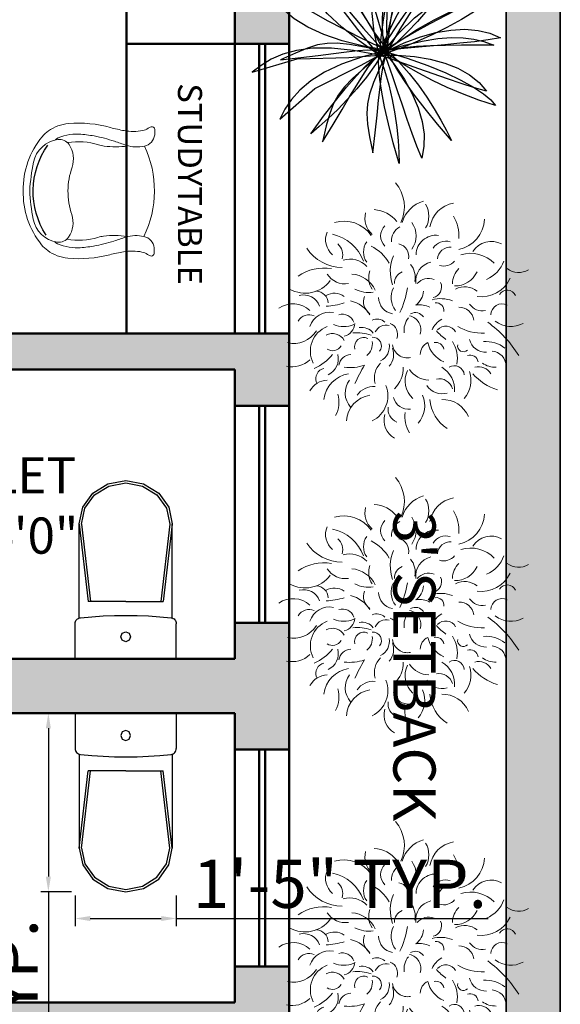
# Model space of a CAD drawing. Units: inches. Extents: x 2442 to 3851, y 589 to 2836.
# Tile 9 of 22: x 3004 to 3094, y 1717 to 1880. Entities that reach past the tile are written whole.
import ezdxf

# ---------------------------------------------------------------- set-up
doc = ezdxf.new("R2010")
doc.units = ezdxf.units.IN
for name, color, linetype, lineweight in [('A-ANNO-DIMS', 2, 'Continuous', 18), ('A-ANNO-TEXT', 7, 'Continuous', 18), ('A-AREA-IDEN', 7, 'Continuous', 18), ('A-FLOR-FIXT', 8, 'Continuous', 18), ('A-FURN', 8, 'Continuous', 18), ('A-WALL', 7, 'Continuous', 50), ('A-WALL-PATT', 8, 'Continuous', 13), ('C-PROP', 7, 'Continuous', 35), ('L-PLNT', 94, 'Continuous', 18)]:
    doc.layers.add(name, color=color, linetype=linetype, lineweight=lineweight)
for name, color, linetype in [('DIENHOA', 3, 'Continuous'), ('IFF-FURN-DETAIL', 250, 'Continuous'), ('SANTEH', 7, 'Continuous')]:
    doc.layers.add(name, color=color, linetype=linetype)
doc.styles.add('ATT', font='romans.shx')
doc.styles.get("Standard").update_dxf_attribs({"font": 'arial.ttf'})
doc.dimstyles.new('ISO-25', dxfattribs={"dimtxt": 8, "dimasz": 2.5, "dimexe": 1.25, "dimexo": 0.625, "dimtad": 1, "dimlunit": 3, "dimtxsty": 'Standard', "dimcen": 2.5, "dimadec": 0, "dimazin": 0, "dimtfac": 1, "dimtmove": 0, "dimatfit": 3, "dimfxl": 1, "dimarcsym": 0})

# ---------------------------------------------------------------- blocks, each defined once
blk = doc.blocks.new('ILNG95')
for points in [[(120, 307.8, -0.32971), (50.6, 383.9, -0.036099), (49.5, 421.7, -0.497733), (75, 439.3, -0.070621), (96.1, 428.8, 0.101868), (132.6, 413.5, 0.091794), (258.7, 412, 0.024114), (350.8, 432.5, -0.090294), (637.9, 457.7, -0.132412), (774.5, 407, -0.068618), (816.3, 367.6, -0.184346), (942.9, -0.4, 1.803905)], [(120, 307.8, 0.138132), (243.9, 312.8, 0.001085), (324.6, 339.3, -0.034227), (462.2, 374.6, -0.033255), (566.6, 386.7, -0.137428), (726.9, 350.3, -4.561553)], [(120, 307.8, 0.138132), (243.9, 312.8, 0.001085), (324.6, 339.3, -0.034227), (462.2, 374.6, -0.033255), (566.6, 386.7, -0.137428), (726.9, 350.3, -4.561553)], [(235.1, 307.5, 0.064243), (394.2, 306.7, 0.04414), (433.1, 315, -0.118032), (643, 328.5, -6.296816)], [(235.1, 307.5, 0.064243), (394.2, 306.7, 0.04414), (433.1, 315, -0.118032), (643, 328.5, -6.296816)], [(639.1, -0.4, 0.078302), (611.9, 161.3, -0.233633), (633, 315.1, -0.28763), (710.5, 349.3, -0.317923), (874.6, 193.2, -0.032882), (899.6, 0, 1.140397)], [(639.1, -0.4, 0.078302), (611.9, 161.3, -0.233633), (633, 315.1, -0.28763), (710.5, 349.3, -0.317923), (874.6, 193.2, -0.032882), (899.6, 0, 1.140397)], [(120, -307.8, 0.32971), (50.6, -383.9, 0.036099), (49.5, -421.7, 0.497733), (75, -439.3, 0.070621), (96.1, -428.8, -0.101868), (132.6, -413.5, -0.091794), (258.7, -412, -0.024114), (350.8, -432.5, 0.090294), (637.9, -457.7, 0.132412), (774.5, -407, 0.068618), (816.3, -367.6, 0.184346), (942.9, 0.4, -1.803905)], [(639.1, 0.4, -0.078302), (611.9, -161.3, 0.233633), (633, -315.1, 0.28763), (710.5, -349.3, 0.317923), (874.6, -193.2, 0.032882), (899.6, 0, -1.140397)], [(639.1, 0.4, -0.078302), (611.9, -161.3, 0.233633), (633, -315.1, 0.28763), (710.5, -349.3, 0.317923), (874.6, -193.2, 0.032882), (899.6, 0, -1.140397)], [(120, -307.8, -0.138132), (243.9, -312.8, -0.001085), (324.6, -339.3, 0.034227), (462.2, -374.6, 0.033255), (566.6, -386.7, 0.137428), (726.9, -350.3, 4.561553)], [(120, -307.8, -0.138132), (243.9, -312.8, -0.001085), (324.6, -339.3, 0.034227), (462.2, -374.6, 0.033255), (566.6, -386.7, 0.137428), (726.9, -350.3, 4.561553)], [(235.1, -307.5, -0.064243), (394.2, -306.7, -0.04414), (433.1, -315, 0.118032), (643, -328.5, 6.296816)], [(235.1, -307.5, -0.064243), (394.2, -306.7, -0.04414), (433.1, -315, 0.118032), (643, -328.5, 6.296816)]]:
    blk.add_lwpolyline(points, format="xyb")
blk.add_arc((758.7, 0.8), 708.7, 154.32815, 205.80105)
at = {"layer": 'IFF-FURN-DETAIL'}
blk.add_arc((326.4, -1.7), 549.3, 326.8997, 34.66912, dxfattribs=at)
blk.add_arc((326.4, -1.7), 549.3, 326.8997, 34.66912, dxfattribs=at)
blk = doc.blocks.new('WC 2 Symb_109')
at = {"layer": 'SANTEH'}
for p, q in [((0, 0), (0, 380)), ((0, 380), (132.4, 380)), ((153.6, 364.9), (506.8, 364.9)), ((506.3, 364.9), (215.7, 330.9)), ((506.3, 356), (215.7, 322)), ((215.7, 190), (215.7, 330.9)), ((215.7, 190), (215.7, 49.1)), ((506.3, 24), (215.7, 58)), ((506.3, 15.1), (215.7, 49.1)), ((153.8, 15.1), (506.8, 15.1)), ((0, 0), (132.4, 0))]:
    blk.add_line(p, q, dxfattribs=at)
for points in [[(154.6, 360.1), (153.9, 364.1), (152.3, 367.9), (150.2, 371.3), (147.4, 374.3), (144.1, 376.7), (140.5, 378.5), (136.5, 379.6), (132.4, 380)], [(154.6, 19.7), (158.6, 62.1), (161.4, 104.7), (163.1, 147.3), (163.7, 189.9), (163.1, 232.5), (161.4, 275.1), (158.6, 317.7), (154.6, 360.1)], [(506.3, 24), (565.5, 36.6), (615.7, 72.6), (649.2, 126.5), (661, 190), (649.2, 253.5), (615.7, 307.4), (565.5, 343.4), (506.3, 356)], [(506.8, 15.1), (569.2, 28.4), (622.2, 66.3), (657.6, 123.1), (670, 190), (657.6, 256.9), (622.2, 313.7), (569.2, 351.6), (506.8, 364.9)], [(132.4, 0), (136.5, 0.4), (140.4, 1.5), (144.1, 3.2), (147.3, 5.6), (150.1, 8.6), (152.3, 12), (153.8, 15.7), (154.6, 19.7)]]:
    blk.add_lwpolyline(points, dxfattribs=at)
blk.add_lwpolyline([(83.6, 208.5), (70.4, 203.1), (64.9, 190), (70.4, 176.9), (83.6, 171.5), (96.8, 176.9), (102.2, 190), (96.8, 203.1)], close=True, dxfattribs=at)
blk = doc.blocks.new('12PPLT14')
at = {"color": 0, "linetype": 'ByBlock'}
for centre, radius, start, end in [((-0.1625, 0.4338), 0.1552, 335.4234, 39.9527), ((0.1087, 0.3325), 0.1308, 106.3737, 163.6865), ((0.216, 0.3316), 0.1193, 99.6686, 170.3916), ((-0.0808, 0.3868), 0.0897, 165.5676, 227.7978), ((-0.1402, 0.294), 0.1288, 38.2331, 86.4254), ((-0.0015, 0.3959), 0.0956, 329.2952, 30.7048), ((-0.2571, 0.2399), 0.1351, 34.2662, 106.816), ((-0.0514, 0.3138), 0.0928, 323.3029, 36.6971), ((0.0506, 0.3121), 0.1678, 356.7873, 29.9706), ((0.1909, 0.3893), 0.1338, 281.7312, 357.1257), ((-0.2523, 0.2979), 0.0813, 157.2527, 229.5051), ((-0.0467, 0.3138), 0.0589, 134.2792, 225.7208), ((0.0083, 0.2908), 0.0696, 119.3333, 181.2289), ((-0.3428, 0.1468), 0.1777, 20.6522, 77.761), ((-0.1032, 0.2472), 0.0733, 144.9004, 215.0996), ((0.1238, 0.2336), 0.083, 82.9962, 178.2659), ((0.1649, 0.2288), 0.0631, 73.677, 147.4747), ((0.3529, 0.1986), 0.0923, 62.4899, 146.6083), ((-0.2631, 0.3606), 0.1778, 213.4024, 269.326), ((-0.3207, 0.2361), 0.0583, 342.2672, 49.5918), ((-0.223, 0.1138), 0.1758, 29.5718, 63.8395), ((-0.0403, 0.2301), 0.0513, 346.7243, 78.6914), ((0.1827, 0.2139), 0.0534, 85.265, 175.2671), ((-0.2335, 0.1217), 0.0961, 42.9815, 106.4777), ((0.103, 0.1659), 0.1687, 157.0616, 198.7007), ((0.1187, 0.1278), 0.0788, 101.6359, 188.4366), ((0.1561, 0.2471), 0.0582, 252.2434, 319.6792), ((0.2662, 0.1039), 0.1379, 44.5227, 106.5076), ((0.2843, 0.2512), 0.1271, 292.7233, 340.8083), ((-0.3406, -0.0039), 0.1849, 80.336, 125.1387), ((-0.071, 0.1405), 0.0841, 159.833, 213.5727), ((0.002, 0.1188), 0.05, 112.1748, 182.9374), ((-0.0525, 0.1406), 0.0902, 350.0819, 37.9622), ((0.2797, 0.1152), 0.0882, 134.2975, 179.349), ((0.2042, 0.2053), 0.098, 267.7941, 335.7788), ((0.4652, 0.2401), 0.0779, 232.4069, 301.8623), ((-0.4178, 0.2048), 0.1282, 239.7244, 324.0772), ((-0.2521, 0.2046), 0.0894, 212.7771, 278.7223), ((-0.2353, 0.0367), 0.1199, 26.1776, 85.1926), ((0.094, 0.072), 0.0659, 70.3325, 137.7683), ((0.3092, 0.1973), 0.1353, 263.3454, 334.185), ((-0.3739, 0.0341), 0.0511, 2.467, 87.4728), ((-0.1543, 0.2003), 0.1209, 241.5287, 278.4347), ((0.0228, 0.0586), 0.0851, 152.0419, 218.8274), ((-0.34, 0.1477), 0.3488, 334.29, 351.8885), ((-0.0111, 0.0925), 0.0832, 308.5351, 354.9136), ((0.1017, 0.1024), 0.045, 282.8815, 24.0365), ((0.2424, 0.0217), 0.0815, 51.1397, 117.4271), ((0.4187, 0.0518), 0.0378, 24.3786, 147.9852), ((-0.4247, -0.0009), 0.0706, 19.8329, 104.6003), ((-0.2974, 0.0074), 0.0691, 53.5126, 119.7474), ((-0.2616, -0.0829), 0.132, 32.2356, 76.0319), ((-0.1183, 0.0408), 0.0581, 157.5609, 237.1128), ((-0.0447, 0.0607), 0.0698, 181.7454, 260.0237), ((0.1427, -0.0803), 0.1346, 68.7259, 105.2422), ((-0.468, -0.0701), 0.1027, 47.2022, 124.8992), ((-0.3432, 0.3083), 0.2855, 272.3147, 287.7219), ((0.0563, -0.0634), 0.0921, 62.7918, 99.6978), ((0.125, 0.0053), 0.0314, 351.8398, 98.1), ((0.2201, -0.0419), 0.0605, 6.851, 91.8869), ((0.3159, 0.0688), 0.0649, 214.6894, 281.6662), ((0.3966, -0.0128), 0.0455, 62.415, 179.5656), ((-0.4019, -0.0635), 0.0512, 65.2631, 151.643), ((-0.3178, -0.086), 0.0842, 78.2859, 162.9253), ((-0.2636, -0.0603), 0.0501, 19.5336, 107.2881), ((-0.1211, -0.079), 0.0486, 46.81, 114.2458), ((0.0687, -0.0762), 0.0776, 139.4669, 188.6741), ((0.0015, -0.0752), 0.0596, 343.1915, 77.687), ((0.0376, -0.0452), 0.0417, 34.8572, 117.0419), ((0.197, -0.1152), 0.0984, 120.3942, 155.6913), ((0.4332, 0.0428), 0.1041, 231.8734, 299.32), ((-0.465, -0.0212), 0.1099, 256.1392, 328.2356), ((-0.2877, -0.1629), 0.109, 111.2663, 206.9249), ((-0.2585, 0.0428), 0.1041, 246.1369, 293.8631), ((-0.2726, -0.0426), 0.0609, 285.5398, 354.9083), ((-0.1835, -0.1238), 0.059, 37.3855, 100.4991), ((-0.0834, -0.1038), 0.0488, 74.167, 155.4291), ((-0.0828, -0.0921), 0.0473, 337.5706, 68.783), ((0.3403, 0.1226), 0.295, 223.1416, 233.5315), ((0.1639, -0.1068), 0.0471, 29.6516, 136.9148), ((0.3131, 0.1083), 0.1966, 239.6382, 273.343), ((0.055, -0.4368), 0.4844, 31.8508, 54.2708), ((-0.3051, -0.1456), 0.0555, 28.564, 118.6243), ((-0.2031, -0.2618), 0.1748, 70.7416, 95.8247), ((-0.1751, -0.1446), 0.0382, 64.5989, 195.0715), ((-0.1379, -0.1412), 0.0356, 321.496, 95.0552), ((0.3301, -0.0984), 0.0696, 193.4793, 272.7231), ((-0.3049, -0.1199), 0.0412, 237.1862, 328.8294), ((-0.1983, -0.1346), 0.0584, 307.0043, 10.961), ((-0.1367, -0.1434), 0.0675, 297.4603, 9.4578), ((-0.1261, -0.1768), 0.0743, 318.9446, 21.0601), ((0.0056, -0.1284), 0.0629, 187.6037, 281.9043), ((0.1122, -0.1766), 0.0537, 114.9911, 180.121), ((0.2021, -0.1018), 0.1155, 193.035, 246.5169), ((0.1228, -0.1611), 0.0339, 11.252, 101.3122), ((0.0954, -0.19), 0.1169, 346.8331, 34.7134), ((0.2371, -0.1417), 0.0239, 167.9887, 313.8509), ((0.3295, -0.2531), 0.1299, 52.4116, 94.1568), ((-0.4721, -0.1203), 0.1079, 257.3279, 313.213), ((-0.4582, -0.0549), 0.1957, 293.3946, 321.4742), ((-0.3545, -0.1945), 0.0737, 295.4172, 13.937), ((-0.2272, -0.2284), 0.0518, 92.735, 171.8723), ((0.265, -0.2125), 0.0333, 8.0854, 109.9339), ((0.3525, -0.2241), 0.0608, 358.6144, 87.0834), ((-0.3303, -0.2772), 0.044, 103.5534, 199.8954), ((-0.2342, -0.0362), 0.1951, 263.4737, 288.5568), ((0.4875, -0.6182), 0.7699, 148.9497, 155.3056), ((-0.0491, -0.2722), 0.0823, 133.2929, 197.2496), ((-0.1342, -0.2328), 0.1218, 315.1067, 1.332), ((0.0958, -0.2858), 0.1, 154.8808, 226.8679), ((0.0984, -0.1813), 0.1021, 214.3427, 267.4969), ((0.0948, -0.3222), 0.106, 354.6407, 60.4156), ((0.2004, -0.2632), 0.04, 3.1298, 123.6919), ((0.3002, -0.2876), 0.0597, 31.279, 105.0766), ((0.3711, -0.1347), 0.0953, 234.4297, 271.3309), ((-0.3258, -0.3645), 0.0813, 91.0528, 153.0122), ((-0.2197, -0.3768), 0.1216, 98.9327, 173.5652), ((-0.1666, -0.3361), 0.0858, 141.9374, 222.639), ((0.137, -0.3342), 0.0567, 15.8404, 102.1789), ((0.1534, -0.2836), 0.1149, 319.1908, 18.2125), ((0.4504, -0.1006), 0.2342, 221.7868, 251.9354), ((-0.1356, -0.3909), 0.0814, 84.4526, 145.9961), ((-0.1912, -0.3476), 0.1157, 295.6702, 21.368), ((0.1487, -0.2627), 0.0766, 213.8932, 285.618), ((-0.4022, -0.3739), 0.1237, 333.1557, 15.4351), ((-0.1321, -0.4596), 0.1156, 98.8586, 176.1805), ((0.0095, -0.3403), 0.0634, 192.7121, 278.2146), ((-0.0287, -0.3897), 0.1058, 317.7735, 24.7522), ((0.2528, -0.3527), 0.1547, 183.8744, 237.3741), ((0.1506, -0.4799), 0.1168, 23.0406, 91.6662), ((-0.0165, -0.4023), 0.0586, 172.0702, 247.3677), ((-0.0081, -0.4497), 0.0833, 162.968, 241.4878), ((0.1108, -0.4364), 0.1161, 170.0959, 213.6572)]:
    blk.add_arc(centre, radius, start, end, dxfattribs=at)
at = {"color": 0, "linetype": 'ByBlock', "style": 'ATT'}
for tag, p, flags in [('ITEM', (-1.4111, -3.0457), 3), ('ROOM_NUMBER', (-1.4111, -4.379), 1)]:
    blk.add_attdef(tag, p, '', height=1, dxfattribs=dict(at, flags=flags))
blk = doc.blocks.new('Cay03_mb')
at = {"layer": 'DIENHOA'}
for p, q in [((118.6, 555.3), (166.2, 599.1)), ((166.2, 599.1), (142.2, 519.4)), ((79.5, 503.7), (118.6, 555.3)), ((48.6, 443.6), (79.5, 503.7)), ((142.2, 519.4), (119, 441.7)), ((25.5, 374.3), (48.6, 443.6)), ((119, 441.7), (96.7, 365.6)), ((-365.2, 390.3), (-414.4, 402.8)), ((-414.4, 402.8), (-240.2, 277.8)), ((-314.9, 371.3), (-365.2, 390.3)), ((-263.5, 343.5), (-314.9, 371.3)), ((9.9, 295.3), (25.5, 374.3)), ((96.7, 365.6), (75.6, 290.6)), ((-211.2, 304.6), (-263.5, 343.5)), ((-240.2, 277.8), (-88.4, 94.9)), ((-158, 252.3), (-211.2, 304.6)), ((1.6, 205.7), (9.9, 295.3)), ((75.6, 290.6), (55.7, 216.3)), ((290.6, 243.2), (363.4, 275.4)), ((363.4, 275.4), (436.8, 297.2)), ((436.8, 297.2), (511, 309.6)), ((511.8, 271.4), (437.6, 231.5)), ((511, 309.6), (585.9, 313.5)), ((585.9, 313.5), (511.8, 271.4)), ((-104.2, 184.4), (-158, 252.3)), ((218.5, 199.8), (290.6, 243.2)), ((437.6, 231.5), (363.7, 192.9)), ((-49.6, 98.5), (-104.2, 184.4)), ((0.2, 104.9), (1.6, 205.7)), ((55.7, 216.3), (37.3, 142.1)), ((147, 144.1), (218.5, 199.8)), ((363.7, 192.9), (290.2, 154.9)), ((37.3, 142.1), (20.5, 67.6)), ((75.9, 75.2), (147, 144.1)), ((290.2, 154.9), (217.4, 116.6)), ((-88.4, 94.9), (5.4, -7.8)), ((5.4, -7.8), (-49.6, 98.5)), ((5.4, -7.8), (0.2, 104.9)), ((217.4, 116.6), (145.5, 77.3)), ((5.4, -7.8), (75.9, 75.2)), ((20.5, 67.6), (5.4, -7.8)), ((145.5, 77.3), (74.7, 36.1)), ((182.2, 37.2), (253, 48.9)), ((253, 48.9), (314.6, 54.1)), ((314.6, 54.1), (369.2, 53.3)), ((369.2, 53.3), (418.6, 46.8)), ((418.6, 46.8), (464.9, 35.2)), ((-345, 5.4), (-399.6, -17.1)), ((-298.6, 20.1), (-345, 5.4)), ((-254.7, 27.4), (-298.6, 20.1)), ((-208, 27.8), (-254.7, 27.4)), ((-152.7, 21.7), (-208, 27.8)), ((-83.4, 9.7), (-152.7, 21.7)), ((5.4, -7.8), (-83.4, 9.7)), ((74.7, 36.1), (5.4, -7.8)), ((5.4, -7.8), (100.3, 18.4)), ((46.3, 0.9), (5.4, -7.8)), ((96.7, 7.5), (46.3, 0.9)), ((155, 12.2), (96.7, 7.5)), ((100.3, 18.4), (182.2, 37.2)), ((219.6, 15.4), (155, 12.2)), ((289, 17.4), (219.6, 15.4)), ((361.6, 18.5), (289, 17.4)), ((435.8, 18.9), (361.6, 18.5)), ((510, 19), (435.8, 18.9)), ((464.9, 35.2), (510, 19)), ((-399.6, -17.1), (-468, -47.9)), ((-468, -47.9), (-375.6, -37.8)), ((-375.6, -37.8), (-295.3, -27.9)), ((-295.3, -27.9), (-225.8, -18.9)), ((-225.8, -18.9), (-165.8, -11.3)), ((-165.8, -11.3), (-114, -5.7)), ((-114, -5.7), (-69, -2.9)), ((-69, -2.9), (-29.6, -3.4)), ((-45.1, -46.3), (-16.5, -22.4)), ((5.4, -7.8), (-33.2, -69.5)), ((-29.6, -3.4), (5.4, -7.8)), ((-16.5, -22.4), (5.4, -7.8)), ((5.4, -7.8), (56.8, -73.3)), ((25.9, -64.4), (5.4, -7.8)), ((5.4, -7.8), (112.8, -40.3)), ((53.5, -41.6), (5.4, -7.8)), ((107, -75.7), (53.5, -41.6)), ((112.8, -40.3), (207.5, -73.8)), ((-120.2, -122.1), (-79.8, -79.6)), ((-79.8, -79.6), (-45.1, -46.3)), ((-33.2, -69.5), (-74.6, -127.3)), ((47, -125.9), (25.9, -64.4)), ((56.8, -73.3), (100.4, -139.1)), ((165.5, -109.6), (107, -75.7)), ((207.5, -73.8), (289.5, -107.6)), ((-165.9, -174.1), (-120.2, -122.1)), ((-74.6, -127.3), (-117.8, -181.1)), ((68.7, -190.6), (47, -125.9)), ((228.7, -142.8), (165.5, -109.6)), ((289.5, -107.6), (359.3, -141.1)), ((-216.3, -235.6), (-165.9, -174.1)), ((100.4, -139.1), (135.9, -204.3)), ((296, -174.7), (228.7, -142.8)), ((367.1, -204.8), (296, -174.7)), ((359.3, -141.1), (416.9, -173.5)), ((416.9, -173.5), (462.6, -204.2)), ((-117.8, -181.1), (-162.1, -230.9)), ((90.8, -256.6), (68.7, -190.6)), ((135.9, -204.3), (162.8, -268.3)), ((441.6, -232.7), (367.1, -204.8)), ((462.6, -204.2), (496.5, -232.5)), ((-271, -306.6), (-216.3, -235.6)), ((-162.1, -230.9), (-206.3, -276.5)), ((113.1, -322.2), (90.8, -256.6)), ((162.8, -268.3), (181, -330.4)), ((518.9, -257.7), (441.6, -232.7)), ((496.5, -232.5), (518.9, -257.7)), ((-329.5, -387.1), (-271, -306.6)), ((-206.3, -276.5), (-249.6, -317.8)), ((-291, -354.7), (-329.5, -387.1)), ((-249.6, -317.8), (-291, -354.7)), ((135.4, -385.6), (113.1, -322.2)), ((181, -330.4), (190, -390)), ((157.6, -445), (135.4, -385.6)), ((190, -390), (189.6, -446.3)), ((179.5, -498.7), (157.6, -445)), ((189.6, -446.3), (179.5, -498.7))]:
    blk.add_line(p, q, dxfattribs=at)
for points in [[(23.7, -5.4), (-41, 82.2), (-91.8, 167.1), (-129.7, 249.5), (-155.6, 329.6), (-170.2, 407.8), (-174.7, 484.2), (-169.8, 559.3), (-156.5, 633.1)], [(-156.5, 633.1), (-132.5, 551.3), (-110.5, 470), (-89.8, 389.2), (-69.6, 309), (-49, 229.4), (-27.1, 150.4), (-3.2, 72.1), (23.7, -5.4)], [(-16.4, -26.7), (-38.3, 80), (-48.9, 178.3), (-48.7, 269), (-38.5, 352.6), (-19.1, 429.7), (9, 501), (44.9, 567.1), (87.9, 628.5)], [(87.9, 628.5), (75.5, 544.2), (61.3, 461.2), (46.1, 379.1), (30.8, 297.8), (16.1, 216.9), (2.9, 136), (-8.3, 54.9), (-16.4, -26.7)], [(-395.6, 473.7), (-347.5, 405.6), (-300.6, 339.5), (-254.3, 275.1), (-208.3, 212.3), (-161.9, 150.9), (-114.8, 90.7), (-66.5, 31.6), (-16.4, -26.7)], [(-16.4, -26.7), (-108.3, 38.6), (-186.9, 101.7), (-252.4, 163.5), (-305.1, 224.4), (-345.4, 285.2), (-373.7, 346.6), (-390.4, 409.2), (-395.6, 473.7)], [(23.7, -5.4), (19.8, 93), (20.3, 177), (25, 248.5), (34, 309.8), (47.3, 362.7), (64.9, 409.3), (86.8, 451.7), (112.9, 491.9)], [(112.9, 491.9), (96, 419.7), (79.5, 347.4), (63.9, 276.5), (50, 208.4), (38.4, 144.8), (29.7, 86.9), (24.6, 36.3), (23.7, -5.4)], [(384.3, 437.5), (342.2, 367.8), (298.1, 301.7), (252.6, 239.4), (206.1, 181.1), (159.4, 127.2), (113, 78), (67.6, 33.6), (23.7, -5.4)], [(23.7, -5.4), (79.9, 91.7), (134.1, 176.2), (185.8, 248.4), (234.3, 308.7), (279, 357.3), (319.3, 394.8), (354.6, 421.4), (384.3, 437.5)], [(273.2, 387.3), (227.6, 328.8), (182.3, 270.1), (138.4, 212.3), (97.2, 156.4), (60, 103.4), (27.8, 54.6), (1.9, 10.8), (-16.4, -26.7)], [(-16.4, -26.7), (21.4, 64.2), (57, 140.3), (91.4, 203.3), (125.2, 255.1), (159.5, 297.5), (195, 332.5), (232.7, 361.8), (273.2, 387.3)], [(-530.5, 289.7), (-458.3, 248.1), (-387.9, 207.8), (-318.9, 168.7), (-250.8, 131.1), (-182.9, 94.8), (-114.9, 59.9), (-46.2, 26.5), (23.7, -5.4)], [(23.7, -5.4), (-87.2, 15.2), (-185, 39.6), (-270.3, 68.2), (-343.7, 101.4), (-405.9, 139.7), (-457.3, 183.5), (-498.7, 233.4), (-530.5, 289.7)], [(496.7, 224), (429.4, 178.4), (361.6, 136.9), (294.1, 99.5), (227.5, 66.1), (162.4, 36.7), (99.7, 11.5), (39.8, -9.7), (-16.4, -26.7)], [(-16.4, -26.7), (75.4, 37.9), (160.1, 91.8), (237.3, 135.7), (306.6, 170), (367.6, 195.4), (419.9, 212.5), (463.1, 221.9), (496.7, 224)], [(23.7, -5.4), (99.3, 29.7), (173.2, 57.1), (244.8, 76.7), (313.3, 88.3), (377.9, 91.8), (437.9, 87), (492.7, 73.8), (541.4, 52)], [(541.4, 52), (484.1, 42.9), (421.2, 34.8), (354.4, 27.6), (285.4, 20.9), (216.1, 14.5), (148.2, 8.1), (83.5, 1.6), (23.7, -5.4)], [(-16.4, -26.7), (-134, -4.7), (-235.3, 5.3), (-322, 4.7), (-395.9, -5), (-458.7, -22.3), (-512.3, -45.7), (-558.2, -73.6), (-598.4, -104.7)], [(-598.4, -104.7), (-392.7, -44.4), (-155, -37.4), (-16.4, -26.7)], [(-471.9, -320.3), (-310.5, -179.3), (-97.7, -73.3), (23.7, -5.4)], [(23.7, -5.4), (-92.3, -34.8), (-188.4, -68.2), (-266.9, -105.1), (-329.9, -144.9), (-379.7, -187), (-418.5, -230.7), (-448.5, -275.3), (-471.9, -320.3)], [(-276.2, -424.4), (-227.3, -345.4), (-185.7, -276.1), (-150, -215.7), (-119.1, -163.8), (-91.5, -119.5), (-66, -82.3), (-41.4, -51.6), (-16.4, -26.7)], [(-16.4, -26.7), (-84.9, -86), (-137, -133.1), (-175.8, -173), (-204.3, -210), (-225.5, -249.1), (-242.5, -294.7), (-258.4, -351.6), (-276.2, -424.4)], [(23.7, -5.4), (-13.6, -87.9), (-41.1, -152.6), (-59.6, -205), (-69.9, -250.7), (-72.8, -295), (-69.2, -343.6), (-59.7, -401.9), (-45.3, -475.5)], [(-45.3, -475.5), (-34.1, -383.2), (-25.4, -302.8), (-18.3, -233.1), (-12, -172.9), (-5.6, -121.2), (2, -76.8), (11.4, -38.5), (23.7, -5.4)], [(76.2, -524.2), (48.8, -428.5), (26.6, -341.7), (9.2, -264.1), (-3.6, -196.1), (-12.3, -138), (-17.1, -90.2), (-18.3, -53), (-16.4, -26.7)], [(-16.4, -26.7), (66.9, -26.6), (145.6, -32.7), (218.8, -44.9), (285.8, -63.1), (345.9, -87.1), (398.4, -116.6), (442.6, -151.6), (477.6, -191.8)], [(477.6, -191.8), (421.8, -176), (361.3, -156.9), (297.6, -135.5), (232.2, -112.6), (166.6, -89.4), (102.3, -66.6), (40.8, -45.4), (-16.4, -26.7)], [(-16.4, -26.7), (8.5, -95.1), (28.5, -163.3), (44.3, -230.6), (56.3, -296.1), (65, -359), (70.9, -418.5), (74.5, -473.9), (76.2, -524.2)], [(316.5, -418.1), (251.4, -342.8), (194.8, -273.3), (146.5, -210.2), (106.3, -153.8), (74.1, -104.7), (49.7, -63.4), (32.9, -30.1), (23.7, -5.4)], [(23.7, -5.4), (74.9, -57.1), (121.8, -110.6), (164.3, -165), (202.7, -219.4), (237, -272.9), (267.3, -324.5), (293.7, -373.2), (316.5, -418.1)]]:
    blk.add_lwpolyline(points, dxfattribs=at)
blk = doc.blocks.new('*D156')
at = {"layer": 'A-ANNO-DIMS', "color": 0, "lineweight": -2, "transparency": 16777216}
for p, q in [((3012.46, 1764.86), (3007.39, 1764.86)), ((3008.64, 1762.36), (3008.64, 1737.76)), ((3012.46, 1735.26), (3007.39, 1735.26)), ((3008.64, 1735.26), (3008.64, 1642.05))]:
    blk.add_line(p, q, dxfattribs=at)
at = {"layer": 'A-ANNO-DIMS', "color": 0, "transparency": 16777216}
for points in [[(3008.22, 1762.36), (3009.06, 1762.36), (3008.64, 1764.86)], [(3008.22, 1737.76), (3009.06, 1737.76), (3008.64, 1735.26)]]:
    blk.add_solid(points, dxfattribs=at)
at = {"layer": 'Defpoints', "color": 0, "transparency": 16777216}
for p in [(3013.08, 1764.86), (3008.64, 1735.26), (3013.08, 1735.26)]:
    blk.add_point(p, dxfattribs=at)
at = {"layer": 'A-ANNO-DIMS', "color": 0, "transparency": 16777216, "insert": (3003.88, 1687.4), "char_height": 8, "attachment_point": 5, "rotation": 90}
blk.add_mtext('WC 2\'-5 1/2" TYP.', dxfattribs=at)
blk = doc.blocks.new('*D157')
at = {"layer": 'A-ANNO-DIMS', "color": 0, "lineweight": -2, "transparency": 16777216}
for p, q in [((3013.08, 1734.63), (3013.08, 1729.57)), ((3029.87, 1734.63), (3029.87, 1729.57)), ((3015.58, 1730.82), (3027.37, 1730.82)), ((3029.87, 1730.82), (3081.64, 1730.82))]:
    blk.add_line(p, q, dxfattribs=at)
at = {"layer": 'A-ANNO-DIMS', "color": 0, "transparency": 16777216}
for points in [[(3015.58, 1731.23), (3015.58, 1730.4), (3013.08, 1730.82)], [(3027.37, 1731.23), (3027.37, 1730.4), (3029.87, 1730.82)]]:
    blk.add_solid(points, dxfattribs=at)
at = {"layer": 'Defpoints', "color": 0, "transparency": 16777216}
for p in [(3013.08, 1735.26), (3029.87, 1735.26), (3029.87, 1730.82)]:
    blk.add_point(p, dxfattribs=at)
at = {"layer": 'A-ANNO-DIMS', "color": 0, "transparency": 16777216, "insert": (3057.01, 1735.53), "char_height": 8, "attachment_point": 5}
blk.add_mtext('1\'-5" TYP.', dxfattribs=at)

msp = doc.modelspace()

# ---------------------------------------------------------------- hatches: boundary and pattern name
at = {"layer": 'A-WALL-PATT'}
h = msp.add_hatch(color=256, dxfattribs=at)
h.dxf.hatch_style = 1
h.paths.add_polyline_path([(2502.599, 1992.864), (2719.571, 1992.864), (2719.687, 1994.649), (2720.167, 1997.319), (2721.479, 1992.864), (2726.325, 1992.864), (2727.448, 1994.93), (2729.005, 1997.153), (2728.372, 1992.864), (2728.871, 1992.864), (2730.114, 1994.505), (2731.833, 1996.09), (2730.966, 1993.206), (2730.864, 1992.864), (2771.772, 1992.864), (2771.887, 1994.649), (2772.368, 1997.319), (2773.68, 1992.864), (2778.526, 1992.864), (2779.649, 1994.93), (2781.206, 1997.153), (2780.572, 1992.864), (2781.072, 1992.864), (2782.315, 1994.505), (2784.034, 1996.09), (2783.167, 1993.206), (2783.065, 1992.864), (2821.282, 1992.864), (2821.398, 1994.649), (2821.878, 1997.319), (2823.19, 1992.864), (2828.036, 1992.864), (2829.159, 1994.93), (2830.716, 1997.153), (2830.083, 1992.864), (2830.582, 1992.864), (2831.825, 1994.505), (2833.544, 1996.09), (2832.677, 1993.206), (2832.575, 1992.864), (2869.287, 1992.864), (2869.403, 1994.649), (2869.884, 1997.319), (2871.195, 1992.864), (2876.042, 1992.864), (2877.165, 1994.93), (2878.721, 1997.153), (2878.088, 1992.864), (2878.587, 1992.864), (2879.83, 1994.505), (2881.55, 1996.09), (2880.682, 1993.206), (2880.58, 1992.864), (2919.335, 1992.864), (2919.451, 1994.649), (2919.932, 1997.319), (2921.243, 1992.864), (2926.09, 1992.864), (2927.213, 1994.93), (2928.77, 1997.153), (2928.136, 1992.864), (2928.635, 1992.864), (2929.878, 1994.505), (2931.598, 1996.09), (2930.73, 1993.206), (2930.628, 1992.864), (2966.155, 1992.864), (2966.27, 1994.649), (2966.751, 1997.319), (2968.063, 1992.864), (2972.909, 1992.864), (2974.032, 1994.93), (2975.589, 1997.153), (2974.955, 1992.864), (2975.455, 1992.864), (2976.698, 1994.505), (2978.417, 1996.09), (2977.55, 1993.206), (2977.448, 1992.864), (3010.53, 1992.864), (3010.646, 1994.649), (3011.127, 1997.319), (3012.438, 1992.864), (3017.285, 1992.864), (3018.408, 1994.93), (3019.964, 1997.153), (3019.331, 1992.864), (3019.83, 1992.864), (3021.073, 1994.505), (3022.793, 1996.09), (3021.925, 1993.206), (3021.823, 1992.864), (3057.996, 1992.864), (3058.45, 1995.382), (3059.191, 1992.864), (3065.64, 1992.864), (3067.287, 1995.216), (3066.94, 1992.864), (3068.717, 1992.864), (3070.116, 1994.153), (3069.728, 1992.864), (3084.599, 1992.864), (3084.599, 1983.791), (3085.291, 1983.828), (3084.599, 1983.434), (3084.599, 1932.114), (3085.291, 1932.151), (3084.599, 1931.757), (3084.599, 1886.278), (3085.291, 1886.315), (3084.599, 1885.921), (3084.599, 1410.864), (3066.599, 1410.864), (3066.599, 1401.864), (3093.599, 1401.864), (3093.599, 2001.864), (2493.599, 2001.864), (2493.599, 1401.864), (2538.599, 1401.864), (2538.599, 1410.864), (2502.599, 1410.864)])
h.paths.add_polyline_path([(2738.599, 1410.864), (2547.599, 1410.864), (2547.599, 1401.864), (2738.599, 1401.864)], flags=17)
h.paths.add_polyline_path([(2910.599, 1410.864), (2792.599, 1410.864), (2792.599, 1401.864), (2910.599, 1401.864), (2910.599, 1402.864)], flags=17)
h = msp.add_hatch(color=256, dxfattribs=at)
h.dxf.hatch_style = 1
h.paths.add_polyline_path([(2799.599, 1467.864), (2775.599, 1467.864), (2775.599, 1458.864), (2799.599, 1458.864)])
h.paths.add_polyline_path([(2703.599, 1506.864), (2670.599, 1506.864), (2670.599, 1497.864), (2694.599, 1497.864), (2694.599, 1458.864), (2733.599, 1458.864), (2733.599, 1467.864), (2709.417, 1467.864), (2703.599, 1467.864)])
h.paths.add_polyline_path([(2604.599, 1506.864), (2593.599, 1506.864), (2593.599, 1497.864), (2604.599, 1497.864)])
h.paths.add_polyline_path([(2547.599, 1497.864), (2553.599, 1497.864), (2553.599, 1506.864), (2547.599, 1506.864), (2547.599, 1530.864), (2538.599, 1530.864), (2538.599, 1401.864), (2547.599, 1401.864)])
h.paths.add_polyline_path([(2547.599, 1683.864), (2538.599, 1683.864), (2538.599, 1578.864), (2547.599, 1578.864), (2547.599, 1602.864), (2694.599, 1602.864), (2694.599, 1554.864), (2703.599, 1554.864), (2703.599, 1716.864), (2694.599, 1716.864), (2694.599, 1611.864), (2547.599, 1611.864)])
h.paths.add_polyline_path([(2892.599, 1497.864), (2883.599, 1497.864), (2883.599, 1488.228), (2883.599, 1467.864), (2865.599, 1467.864), (2865.599, 1458.864), (2892.599, 1458.864)])
h.paths.add_polyline_path([(3048.599, 1722.864), (3039.599, 1722.864), (3039.599, 1716.864), (2937.599, 1716.864), (2937.599, 1710.864), (3039.599, 1710.864), (3039.599, 1685.364), (3048.599, 1685.364)])
h.paths.add_polyline_path([(3048.599, 1779.864), (3039.599, 1779.864), (3039.599, 1773.864), (2961.599, 1773.864), (2961.599, 1791.864), (2955.599, 1791.864), (2955.599, 1773.864), (2895.599, 1773.864), (2895.599, 1821.864), (2916.599, 1821.864), (2916.599, 1827.864), (2889.599, 1827.864), (2889.599, 1773.864), (2886.599, 1773.864), (2886.599, 1764.864), (2937.599, 1764.864), (2937.599, 1746.864), (2943.599, 1746.864), (2943.599, 1764.864), (2956.06, 1764.864), (3039.599, 1764.864), (3039.599, 1758.864), (3048.599, 1758.864)])
h.paths.add_polyline_path([(3048.599, 1827.864), (2976.475, 1827.864, -0.1284593), (2975.705, 1827.665), (2964.694, 1827.687, -0.1198794), (2963.972, 1827.864), (2946.599, 1827.864), (2946.599, 1821.864), (3039.599, 1821.864), (3039.599, 1815.864), (3048.599, 1815.864)])
h.paths.add_polyline_path([(3048.599, 1956.864), (3023.366, 1956.864), (3023.277, 1956.402), (3023.088, 1956.864), (3019.494, 1956.864), (3019.543, 1955.479), (3019.146, 1956.864), (3015.599, 1956.864), (3015.599, 1947.864), (3039.599, 1947.864), (3039.599, 1875.864), (3048.599, 1875.864), (3048.599, 1880.743), (3047.576, 1881.614), (3046.081, 1883.417), (3044.931, 1885.453), (3047.541, 1883.949), (3048.599, 1883.343), (3048.599, 1910.588), (3047.049, 1909.235), (3047.896, 1910.862), (3048.599, 1911.909), (3048.599, 1918.826), (3042.477, 1917.032), (3043.928, 1918.154), (3045.59, 1919.165), (3047.525, 1920.009), (3048.599, 1920.305), (3048.599, 1926.579), (3047.576, 1927.45), (3046.081, 1929.252), (3044.931, 1931.289), (3047.541, 1929.785), (3048.599, 1929.179)])
h.paths.add_polyline_path([(2967.599, 1956.864), (2932.171, 1956.864), (2932.082, 1956.402), (2931.893, 1956.864), (2928.299, 1956.864), (2928.348, 1955.479), (2927.951, 1956.864), (2898.599, 1956.864), (2898.599, 1947.864), (2967.599, 1947.864)])
h.paths.add_polyline_path([(2850.599, 1956.864), (2834.118, 1956.864), (2834.029, 1956.402), (2833.84, 1956.864), (2830.245, 1956.864), (2830.294, 1955.479), (2829.897, 1956.864), (2796.599, 1956.864), (2796.599, 1947.864), (2799.599, 1947.864), (2838.599, 1947.864), (2838.599, 1827.864), (2835.599, 1827.864), (2835.599, 1824.864), (2835.599, 1818.864), (2838.599, 1818.864), (2838.599, 1764.864), (2850.599, 1764.864), (2850.599, 1770.864), (2850.599, 1773.864), (2847.599, 1773.864), (2847.599, 1947.864), (2850.599, 1947.864)])
h.paths.add_polyline_path([(2700.599, 1947.864), (2730.599, 1947.864), (2730.599, 1956.864), (2700.599, 1956.864), (2700.599, 1992.864), (2691.599, 1992.864), (2691.599, 1932.864), (2670.599, 1932.864), (2670.599, 1923.864), (2691.599, 1923.864), (2691.599, 1818.864), (2799.599, 1818.864), (2799.599, 1827.864), (2700.599, 1827.864)])
h.paths.add_polyline_path([(2640.599, 1932.864), (2538.599, 1932.864), (2538.599, 1868.364), (2547.599, 1868.364), (2547.599, 1923.864), (2640.599, 1923.864), (2640.599, 1929.864)])
h.paths.add_polyline_path([(2547.599, 1820.364), (2538.599, 1820.364), (2538.599, 1731.864), (2547.599, 1731.864), (2547.599, 1755.864), (2694.599, 1755.864), (2694.599, 1752.864), (2697.599, 1752.864), (2703.599, 1752.864), (2703.599, 1764.864), (2547.599, 1764.864)])
h.paths.add_polyline_path([(2725.858, 1838.187), (2790.115, 1838.187), (2790.115, 1868.602), (2725.858, 1868.602)], flags=25)
h.paths.add_polyline_path([(2892.599, 1671.864), (2883.599, 1671.864), (2883.599, 1563.864), (2892.599, 1563.864), (2892.599, 1602.864), (3048.599, 1602.864), (3048.599, 1637.364), (3039.599, 1637.364), (3039.599, 1611.864), (2892.599, 1611.864)])

# ---------------------------------------------------------------- linework, layer by layer
at = {"layer": 'A-WALL'}
for p, q in [((3048.599, 1602.864), (3048.599, 1956.864)), ((3021.599, 1827.864), (3021.599, 1947.864)), ((3039.599, 1827.864), (3039.599, 1947.864)), ((3021.599, 1875.864), (3048.599, 1875.864)), ((3043.599, 1827.864), (3043.599, 1875.864)), ((3044.599, 1827.864), (3044.599, 1875.864)), ((2946.599, 1827.864), (3048.599, 1827.864)), ((2946.599, 1821.864), (3039.599, 1821.864)), ((3039.599, 1773.864), (3039.599, 1821.864)), ((3039.599, 1815.864), (3048.599, 1815.864)), ((3043.599, 1779.864), (3043.599, 1815.864)), ((3044.599, 1779.864), (3044.599, 1815.864)), ((3039.599, 1779.864), (3048.599, 1779.864)), ((2961.599, 1773.864), (3039.599, 1773.864)), ((2943.599, 1764.864), (3039.599, 1764.864)), ((3039.599, 1716.864), (3039.599, 1764.864)), ((3039.599, 1758.864), (3048.599, 1758.864)), ((3043.599, 1722.864), (3043.599, 1758.864)), ((3044.599, 1722.864), (3044.599, 1758.864)), ((3039.599, 1722.864), (3048.599, 1722.864)), ((2937.599, 1716.864), (3039.599, 1716.864))]:
    msp.add_line(p, q, dxfattribs=at)
at = {"layer": 'C-PROP'}
for points in [[(3066.599, 1401.864), (3093.599, 1401.864), (3093.599, 2001.864), (2493.599, 2001.864), (2493.599, 1401.864), (2738.599, 1401.864)], [(3066.599, 1410.864), (3084.599, 1410.864), (3084.599, 1992.864), (2502.599, 1992.864), (2502.599, 1410.864), (2538.599, 1410.864)]]:
    msp.add_lwpolyline(points, dxfattribs=at)

# ---------------------------------------------------------------- block references
at = {"layer": 'A-FLOR-FIXT', "yscale": 0.0441898926459964, "zscale": 0.0441898926459964}
for p, xscale, rotation in [((3013.083, 1773.864), -0.0441898926459964, 270.0000000000001), ((3013.083, 1764.864), 0.0441898926459964, 269.9999999999999)]:
    msp.add_blockref('WC 2 Symb_109', p, dxfattribs=dict(at, xscale=xscale, rotation=rotation))
at = {"layer": 'A-FURN', "xscale": -0.0243705291132055, "yscale": 0.0243705291132055, "zscale": 0.0243705291132055, "rotation": 359.6824344718516}
msp.add_blockref('ILNG95', (3027.464, 1851.412), dxfattribs=at)
at = {"layer": 'L-PLNT'}
for name, p, xscale, yscale, zscale in [('Cay03_mb', (3064.109, 1874.98), 0.036152509973097, 0.036152509973097, 0.036152509973097), ('12PPLT14', (3068.013, 1831.454), 40.07642696295986, 40.07642696295986, 40.07642696295986), ('12PPLT14', (3068.013, 1782.567), 40.07642696295986, 40.07642696295986, 40.07642696295986), ('12PPLT14', (3068.013, 1725.519), 40.07642696295986, 40.07642696295986, 40.07642696295986)]:
    msp.add_blockref(name, p, dxfattribs=dict(at, xscale=xscale, yscale=yscale, zscale=zscale))

# ---------------------------------------------------------------- texts
at = {"layer": 'A-ANNO-TEXT', "attachment_point": 1, "rotation": 270}
for s, width, heights, insert, char_height in [('{\\fTimes New Roman|b0|i0|c0|p18;STUDYTABLE}', 110.76054, [5.476], (3034.144, 1869.361), 4), ("{\\fTimes New Roman|b0|i0|c0|p18;3' SETBACK}", 79.56037, [0], (3072.895, 1798.403), 7)]:
    msp.add_mtext_dynamic_manual_height_columns(s, width=width, gutter_width=12.5, heights=heights, dxfattribs=dict(at, insert=insert, char_height=char_height))
at = {"layer": 'A-AREA-IDEN', "insert": (2978.437, 1807.325), "char_height": 6, "attachment_point": 1}
msp.add_mtext_dynamic_manual_height_columns('{\\fTimes New Roman|b0|i0|c0|p18;A.TOILET\\P6\'6"X4\'0"}', width=110.76054, gutter_width=12.5, heights=[0], dxfattribs=at)

# ---------------------------------------------------------------- dimensions: what is measured, and where the dimension line sits
at = {"layer": 'A-ANNO-DIMS'}
dim = msp.add_linear_dim(base=(3008.641, 1735.257), p1=(3013.083, 1764.864), p2=(3013.083, 1735.257), angle=270, text='WC <> TYP.', dimstyle='ISO-25', override={"dimdec": 1, "dimrnd": 0, "dimzin": 1, "dimlunit": 4, "dimfrac": 2}, dxfattribs=at)
dim.commit()
dim.dimension.update_dxf_attribs({"geometry": '*D156', "text_midpoint": (3003.88, 1687.403)})
dim = msp.add_linear_dim(base=(3029.875, 1730.816), p1=(3013.083, 1735.257), p2=(3029.875, 1735.257), text='<> TYP.', dimstyle='ISO-25', override={"dimdec": 1, "dimrnd": 0, "dimzin": 1, "dimlunit": 4, "dimfrac": 2}, dxfattribs=at)
dim.commit()
dim.dimension.update_dxf_attribs({"geometry": '*D157', "text_midpoint": (3057.005, 1735.525)})

doc.saveas('drawing.dxf')
